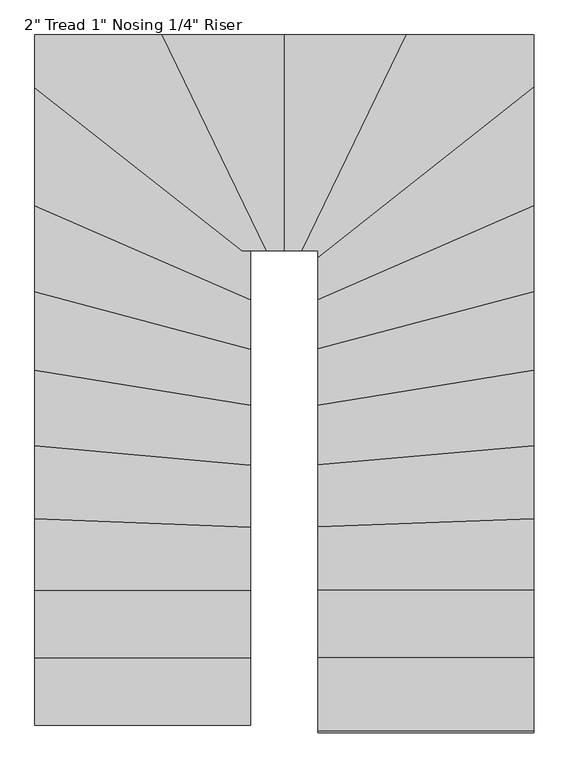
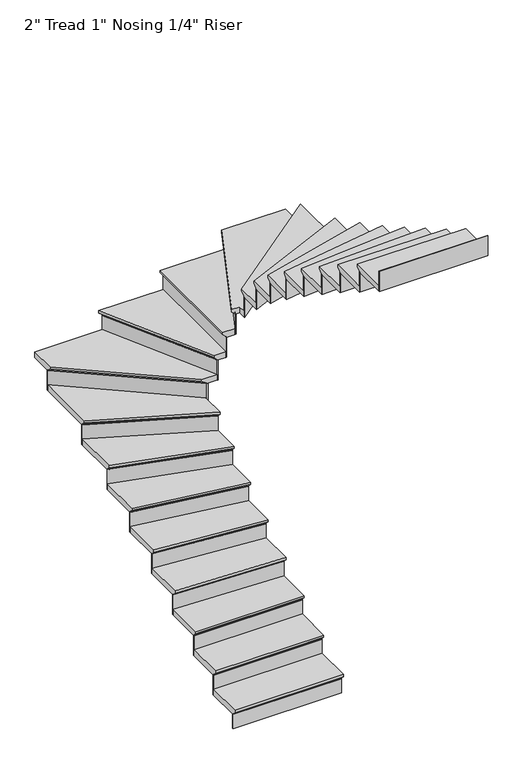
"""IFC4 building model written with IfcOpenShell, lengths in millimetres: stair flight geometry."""

from ifc_helpers import new_model, si_unit, origin, place, context, project, spatial, faceted_brep, source, transform, mapped, element, save


def stair_flight_11ab74ad(model_context):
    return source(origin(), model_context, "Body", "Brep", [
        faceted_brep([(-5047.1987704, -4554.2130548, 51361.5214286), (-5047.1987704, -4554.2130548, 51380.5714286), (-5940.8822214, -4554.2130548, 51380.5714286), (-5940.8822214, -4554.2130548, 51361.5214286), (-5047.1987704, -4528.8130548, 51336.1214286), (-5940.8822214, -4528.8130548, 51336.1214286), (-5047.1987704, -4249.4130548, 51380.5714286), (-5940.8822214, -4249.4130548, 51380.5714286), (-5940.8822214, -4528.8130548, 51329.7714286), (-5940.8822214, -4249.4130548, 51329.7714286), (-5047.1987704, -4249.4130548, 51329.7714286), (-5047.1987704, -4528.8130548, 51329.7714286)], [[[0, 1, 2, 3]], [[4, 0, 3, 5]], [[2, 1, 6, 7]], [[8, 9, 10, 11]], [[2, 7, 9, 8, 5, 3]], [[8, 11, 4, 5]], [[6, 1, 0, 4, 11, 10]], [[7, 6, 10, 9]]]),
        faceted_brep([(-5047.1987704, -4528.8130548, 51329.7714286), (-5047.1987704, -4528.8130548, 51206.4), (-5047.1987704, -4522.4630548, 51206.4), (-5047.1987704, -4522.4630548, 51329.7714286), (-5940.8822214, -4528.8130548, 51329.7714286), (-5940.8822214, -4522.4630548, 51329.7714286), (-5940.8822214, -4522.4630548, 51206.4), (-5940.8822214, -4528.8130548, 51206.4)], [[[0, 1, 2, 3]], [[4, 5, 6, 7]], [[1, 0, 4, 7]], [[2, 1, 7, 6]], [[3, 2, 6, 5]], [[0, 3, 5, 4]]]),
        faceted_brep([(-5047.1987704, -4249.4130548, 51503.9428571), (-5047.1987704, -4249.4130548, 51329.7714286), (-5047.1987704, -4243.0630548, 51329.7714286), (-5047.1987704, -4243.0630548, 51503.9428571), (-5940.8822214, -4249.4130548, 51503.9428571), (-5940.8822214, -4243.0630548, 51503.9428571), (-5940.8822214, -4243.0630548, 51329.7714286), (-5940.8822214, -4249.4130548, 51329.7714286)], [[[0, 1, 2, 3]], [[4, 5, 6, 7]], [[1, 0, 4, 7]], [[2, 1, 7, 6]], [[3, 2, 6, 5]], [[0, 3, 5, 4]]]),
        faceted_brep([(-5940.8822214, -4274.8130548, 51554.7428571), (-5047.1987704, -4274.8130548, 51554.7428571), (-5047.1987704, -3970.0130548, 51554.7428571), (-5940.8822214, -3970.0130548, 51554.7428571), (-5940.8822214, -4249.4130548, 51503.9428571), (-5940.8822214, -3970.0130548, 51503.9428571), (-5047.1987704, -3970.0130548, 51503.9428571), (-5047.1987704, -4249.4130548, 51503.9428571), (-5940.8822214, -4249.4130548, 51510.2928571), (-5940.8822214, -4274.8130548, 51535.6928571), (-5047.1987704, -4249.4130548, 51510.2928571), (-5047.1987704, -4274.8130548, 51535.6928571)], [[[0, 1, 2, 3]], [[4, 5, 6, 7]], [[0, 3, 5, 4, 8, 9]], [[4, 7, 10, 8]], [[2, 1, 11, 10, 7, 6]], [[3, 2, 6, 5]], [[11, 1, 0, 9]], [[10, 11, 9, 8]]]),
        faceted_brep([(-5047.1987704, -3970.0130548, 51678.1142857), (-5047.1987704, -3970.0130548, 51503.9428571), (-5047.1987704, -3963.6630548, 51503.9428571), (-5047.1987704, -3963.6630548, 51678.1142857), (-5940.8822214, -3970.0130548, 51678.1142857), (-5940.8822214, -3963.6630548, 51678.1142857), (-5940.8822214, -3963.6630548, 51503.9428571), (-5940.8822214, -3970.0130548, 51503.9428571)], [[[0, 1, 2, 3]], [[4, 5, 6, 7]], [[1, 0, 4, 7]], [[2, 1, 7, 6]], [[3, 2, 6, 5]], [[0, 3, 5, 4]]]),
        faceted_brep([(-5940.8822214, -3995.4130548, 51728.9142857), (-5047.1987704, -3995.4130548, 51728.9142857), (-5047.1987704, -3707.9036879, 51728.9142857), (-5940.8822214, -3673.2843203, 51728.9142857), (-5940.8822214, -3970.0130548, 51678.1142857), (-5940.8822214, -3673.2843203, 51678.1142857), (-5047.1987704, -3707.9036879, 51678.1142857), (-5047.1987704, -3970.0130548, 51678.1142857), (-5940.8822214, -3970.0130548, 51684.4642857), (-5940.8822214, -3995.4130548, 51709.8642857), (-5047.1987704, -3970.0130548, 51684.4642857), (-5047.1987704, -3995.4130548, 51709.8642857)], [[[0, 1, 2, 3]], [[4, 5, 6, 7]], [[0, 3, 5, 4, 8, 9]], [[4, 7, 10, 8]], [[2, 1, 11, 10, 7, 6]], [[3, 2, 6, 5]], [[11, 1, 0, 9]], [[10, 11, 9, 8]]]),
        faceted_brep([(-5047.1987704, -3707.9036879, 51852.2857143), (-5047.1987704, -3707.9036879, 51678.1142857), (-5047.1987704, -3701.5489252, 51678.1142857), (-5047.1987704, -3701.5489252, 51852.2857143), (-5940.8822214, -3673.2843203, 51852.2857143), (-5940.8822214, -3666.9295576, 51852.2857143), (-5940.8822214, -3666.9295576, 51678.1142857), (-5940.8822214, -3673.2843203, 51678.1142857)], [[[0, 1, 2, 3]], [[4, 5, 6, 7]], [[1, 0, 4, 7]], [[2, 1, 7, 6]], [[3, 2, 6, 5]], [[0, 3, 5, 4]]]),
        faceted_brep([(-5940.8822214, -3698.703371, 51903.0857143), (-5047.1987704, -3733.3227386, 51903.0857143), (-5047.1987704, -3451.3234819, 51903.0857143), (-5940.8822214, -3370.89733, 51903.0857143), (-5940.8822214, -3673.2843203, 51852.2857143), (-5940.8822214, -3370.89733, 51852.2857143), (-5047.1987704, -3451.3234819, 51852.2857143), (-5047.1987704, -3707.9036879, 51852.2857143), (-5940.8822214, -3673.2843203, 51858.6357143), (-5940.8822214, -3698.703371, 51884.0357143), (-5047.1987704, -3707.9036879, 51858.6357143), (-5047.1987704, -3733.3227386, 51884.0357143)], [[[0, 1, 2, 3]], [[4, 5, 6, 7]], [[0, 3, 5, 4, 8, 9]], [[4, 7, 10, 8]], [[2, 1, 11, 10, 7, 6]], [[3, 2, 6, 5]], [[11, 1, 0, 9]], [[10, 11, 9, 8]]]),
        faceted_brep([(-5047.1987704, -3451.3234819, 52026.4571429), (-5047.1987704, -3451.3234819, 51852.2857143), (-5047.1987704, -3444.9478197, 51852.2857143), (-5047.1987704, -3444.9478197, 52026.4571429), (-5940.8822214, -3370.89733, 52026.4571429), (-5940.8822214, -3364.5216678, 52026.4571429), (-5940.8822214, -3364.5216678, 51852.2857143), (-5940.8822214, -3370.89733, 51852.2857143)], [[[0, 1, 2, 3]], [[4, 5, 6, 7]], [[1, 0, 4, 7]], [[2, 1, 7, 6]], [[3, 2, 6, 5]], [[0, 3, 5, 4]]]),
        faceted_brep([(-5940.8822214, -3396.3999789, 52077.2571429), (-5047.1987704, -3476.8261308, 52077.2571429), (-5047.1987704, -3203.4301079, 52077.2571429), (-5940.8822214, -3059.5417727, 52077.2571429), (-5940.8822214, -3370.89733, 52026.4571429), (-5940.8822214, -3059.5417727, 52026.4571429), (-5047.1987704, -3203.4301079, 52026.4571429), (-5047.1987704, -3451.3234819, 52026.4571429), (-5940.8822214, -3370.89733, 52032.8071429), (-5940.8822214, -3396.3999789, 52058.2071429), (-5047.1987704, -3451.3234819, 52032.8071429), (-5047.1987704, -3476.8261308, 52058.2071429)], [[[0, 1, 2, 3]], [[4, 5, 6, 7]], [[0, 3, 5, 4, 8, 9]], [[4, 7, 10, 8]], [[2, 1, 11, 10, 7, 6]], [[3, 2, 6, 5]], [[11, 1, 0, 9]], [[10, 11, 9, 8]]]),
        faceted_brep([(-5047.1987704, -3203.4301079, 52200.6285714), (-5047.1987704, -3203.4301079, 52026.4571429), (-5047.1987704, -3196.9983292, 52026.4571429), (-5047.1987704, -3196.9983292, 52200.6285714), (-5940.8822214, -3059.5417727, 52200.6285714), (-5940.8822214, -3053.109994, 52200.6285714), (-5940.8822214, -3053.109994, 52026.4571429), (-5940.8822214, -3059.5417727, 52026.4571429)], [[[0, 1, 2, 3]], [[4, 5, 6, 7]], [[1, 0, 4, 7]], [[2, 1, 7, 6]], [[3, 2, 6, 5]], [[0, 3, 5, 4]]]),
        faceted_brep([(-5940.8822214, -3085.2688872, 52251.4285714), (-5047.1987704, -3229.1572224, 52251.4285714), (-5047.1987704, -2970.3553609, 52251.4285714), (-5940.8822214, -2732.7052783, 52251.4285714), (-5940.8822214, -3059.5417727, 52200.6285714), (-5940.8822214, -2732.7052783, 52200.6285714), (-5047.1987704, -2970.3553609, 52200.6285714), (-5047.1987704, -3203.4301079, 52200.6285714), (-5940.8822214, -3059.5417727, 52206.9785714), (-5940.8822214, -3085.2688872, 52232.3785714), (-5047.1987704, -3203.4301079, 52206.9785714), (-5047.1987704, -3229.1572224, 52232.3785714)], [[[0, 1, 2, 3]], [[4, 5, 6, 7]], [[0, 3, 5, 4, 8, 9]], [[4, 7, 10, 8]], [[2, 1, 11, 10, 7, 6]], [[3, 2, 6, 5]], [[11, 1, 0, 9]], [[10, 11, 9, 8]]]),
        faceted_brep([(-5047.1987704, -2970.3553609, 52374.8), (-5047.1987704, -2970.3553609, 52200.6285714), (-5047.1987704, -2963.7846771, 52200.6285714), (-5047.1987704, -2963.7846771, 52374.8), (-5940.8822214, -2732.7052783, 52374.8), (-5940.8822214, -2726.1345945, 52374.8), (-5940.8822214, -2726.1345945, 52200.6285714), (-5940.8822214, -2732.7052783, 52200.6285714)], [[[0, 1, 2, 3]], [[4, 5, 6, 7]], [[1, 0, 4, 7]], [[2, 1, 7, 6]], [[3, 2, 6, 5]], [[0, 3, 5, 4]]]),
        faceted_brep([(-5940.8822214, -2758.9880136, 52425.6), (-5047.1987704, -2996.6380961, 52425.6), (-5047.1987704, -2765.8050203, 52425.6), (-5940.8822214, -2375.5896532, 52425.6), (-5940.8822214, -2732.7052783, 52374.8), (-5940.8822214, -2375.5896532, 52374.8), (-5047.1987704, -2765.8050203, 52374.8), (-5047.1987704, -2970.3553609, 52374.8), (-5940.8822214, -2732.7052783, 52381.15), (-5940.8822214, -2758.9880136, 52406.55), (-5047.1987704, -2970.3553609, 52381.15), (-5047.1987704, -2996.6380961, 52406.55)], [[[0, 1, 2, 3]], [[4, 5, 6, 7]], [[0, 3, 5, 4, 8, 9]], [[4, 7, 10, 8]], [[2, 1, 11, 10, 7, 6]], [[3, 2, 6, 5]], [[11, 1, 0, 9]], [[10, 11, 9, 8]]]),
        faceted_brep([(-5047.1987704, -2765.8050203, 52548.9714286), (-5047.1987704, -2765.8050203, 52374.8), (-5047.1987704, -2758.8760908, 52374.8), (-5047.1987704, -2758.8760908, 52548.9714286), (-5940.8822214, -2375.5896532, 52548.9714286), (-5940.8822214, -2368.6607237, 52548.9714286), (-5940.8822214, -2368.6607237, 52374.8), (-5940.8822214, -2375.5896532, 52374.8)], [[[0, 1, 2, 3]], [[4, 5, 6, 7]], [[1, 0, 4, 7]], [[2, 1, 7, 6]], [[3, 2, 6, 5]], [[0, 3, 5, 4]]]),
        faceted_brep([(-5940.8822214, -2403.3053713, 52599.7714286), (-5047.1987704, -2793.5207384, 52599.7714286), (-5047.1987704, -2590.8424524, 52599.7714286), (-5040.8038639, -2590.8424524, 52599.7714286), (-5940.8822214, -1882.1944717, 52599.7714286), (-5940.8822214, -2375.5896532, 52548.9714286), (-5940.8822214, -1882.1944717, 52548.9714286), (-5040.8038639, -2590.8424524, 52548.9714286), (-5047.1987704, -2590.8424524, 52548.9714286), (-5047.1987704, -2765.8050203, 52548.9714286), (-5940.8822214, -2375.5896532, 52555.3214286), (-5940.8822214, -2403.3053713, 52580.7214286), (-5047.1987704, -2765.8050203, 52555.3214286), (-5047.1987704, -2793.5207384, 52580.7214286)], [[[0, 1, 2, 3, 4]], [[5, 6, 7, 8, 9]], [[0, 4, 6, 5, 10, 11]], [[5, 9, 12, 10]], [[2, 1, 13, 12, 9, 8]], [[4, 3, 7, 6]], [[13, 1, 0, 11]], [[12, 13, 11, 10]], [[3, 2, 8, 7]]]),
        faceted_brep([(-5040.8038639, -2590.8424524, 52723.1428571), (-5040.8038639, -2590.8424524, 52548.9714286), (-5030.5387554, -2590.8424524, 52548.9714286), (-5030.5387554, -2590.8424524, 52723.1428571), (-5940.8822214, -1882.1944717, 52723.1428571), (-5940.8822214, -1874.1125661, 52723.1428571), (-5940.8822214, -1874.1125661, 52548.9714286), (-5940.8822214, -1882.1944717, 52548.9714286)], [[[0, 1, 2, 3]], [[4, 5, 6, 7]], [[1, 0, 4, 7]], [[2, 1, 7, 6]], [[3, 2, 6, 5]], [[0, 3, 5, 4]]]),
        faceted_brep([(-5384.6489457, -1697.1590014, 52773.9428571), (-5940.8822214, -1697.1590014, 52773.9428571), (-5940.8822214, -1914.5220945, 52773.9428571), (-5081.8642978, -2590.8424524, 52773.9428571), (-4952.3566185, -2590.8424524, 52773.9428571), (-5940.8822214, -1697.1590014, 52723.1428571), (-5384.6489457, -1697.1590014, 52723.1428571), (-4952.3566185, -2590.8424524, 52723.1428571), (-5040.8038639, -2590.8424524, 52723.1428571), (-5940.8822214, -1882.1944717, 52723.1428571), (-5940.8822214, -1882.1944717, 52729.4928571), (-5940.8822214, -1914.5220945, 52754.8928571), (-5040.8038639, -2590.8424524, 52729.4928571), (-5081.8642978, -2590.8424524, 52754.8928571)], [[[0, 1, 2, 3, 4]], [[5, 6, 7, 8, 9]], [[1, 0, 6, 5]], [[2, 1, 5, 9, 10, 11]], [[9, 8, 12, 10]], [[4, 3, 13, 12, 8, 7]], [[0, 4, 7, 6]], [[13, 3, 2, 11]], [[12, 13, 11, 10]]]),
        faceted_brep([(-4952.3566185, -2590.8424524, 52897.3142857), (-4952.3566185, -2590.8424524, 52723.1428571), (-4945.3027294, -2590.8424524, 52723.1428571), (-4945.3027294, -2590.8424524, 52897.3142857), (-5384.6489457, -1697.1590014, 52897.3142857), (-5377.5950566, -1697.1590014, 52897.3142857), (-5377.5950566, -1697.1590014, 52723.1428571), (-5384.6489457, -1697.1590014, 52723.1428571)], [[[0, 1, 2, 3]], [[4, 5, 6, 7]], [[1, 0, 4, 7]], [[2, 1, 7, 6]], [[3, 2, 6, 5]], [[0, 3, 5, 4]]]),
        faceted_brep([(-5412.8645022, -1697.1590014, 52948.1142857), (-4980.5721749, -2590.8424524, 52948.1142857), (-4882.0987704, -2590.8424524, 52948.1142857), (-4882.0987706, -1697.1590014, 52948.1142857), (-5384.6489457, -1697.1590014, 52897.3142857), (-4882.0987706, -1697.1590014, 52897.3142857), (-4882.0987704, -2590.8424524, 52897.3142857), (-4952.3566185, -2590.8424524, 52897.3142857), (-5384.6489457, -1697.1590014, 52903.6642857), (-5412.8645022, -1697.1590014, 52929.0642857), (-4952.3566185, -2590.8424524, 52903.6642857), (-4980.5721749, -2590.8424524, 52929.0642857)], [[[0, 1, 2, 3]], [[4, 5, 6, 7]], [[0, 3, 5, 4, 8, 9]], [[4, 7, 10, 8]], [[3, 2, 6, 5]], [[11, 1, 0, 9]], [[10, 11, 9, 8]], [[2, 1, 11, 10, 7, 6]]]),
        faceted_brep([(-4882.0987704, -2590.8424524, 53071.4857143), (-4882.0987704, -2590.8424524, 52897.3142857), (-4875.7487704, -2590.8424524, 52897.3142857), (-4875.7487704, -2590.8424524, 53071.4857143), (-4882.0987706, -1697.1590014, 53071.4857143), (-4875.7487706, -1697.1590014, 53071.4857143), (-4875.7487706, -1697.1590014, 52897.3142857), (-4882.0987706, -1697.1590014, 52897.3142857)], [[[0, 1, 2, 3]], [[4, 5, 6, 7]], [[1, 0, 4, 7]], [[2, 1, 7, 6]], [[3, 2, 6, 5]], [[0, 3, 5, 4]]]),
        faceted_brep([(-4907.4987706, -1697.1590014, 53122.2857143), (-4907.4987704, -2590.8424524, 53122.2857143), (-4806.2098095, -2590.8424524, 53122.2857143), (-4373.9174828, -1697.1590014, 53122.2857143), (-4882.0987706, -1697.1590014, 53071.4857143), (-4373.9174828, -1697.1590014, 53071.4857143), (-4806.2098095, -2590.8424524, 53071.4857143), (-4882.0987704, -2590.8424524, 53071.4857143), (-4882.0987706, -1697.1590014, 53077.8357143), (-4907.4987706, -1697.1590014, 53103.2357143), (-4882.0987704, -2590.8424524, 53077.8357143), (-4907.4987704, -2590.8424524, 53103.2357143)], [[[0, 1, 2, 3]], [[4, 5, 6, 7]], [[0, 3, 5, 4, 8, 9]], [[4, 7, 10, 8]], [[2, 1, 11, 10, 7, 6]], [[3, 2, 6, 5]], [[11, 1, 0, 9]], [[10, 11, 9, 8]]]),
        faceted_brep([(-4806.2098095, -2590.8424524, 53245.6571429), (-4806.2098095, -2590.8424524, 53071.4857143), (-4799.1559204, -2590.8424524, 53071.4857143), (-4799.1559204, -2590.8424524, 53245.6571429), (-4373.9174828, -1697.1590014, 53245.6571429), (-4366.8635937, -1697.1590014, 53245.6571429), (-4366.8635937, -1697.1590014, 53071.4857143), (-4373.9174828, -1697.1590014, 53071.4857143)], [[[0, 1, 2, 3]], [[4, 5, 6, 7]], [[1, 0, 4, 7]], [[2, 1, 7, 6]], [[3, 2, 6, 5]], [[0, 3, 5, 4]]]),
        faceted_brep([(-3874.1153195, -1946.8497166, 53296.4571429), (-3874.1153195, -1697.1590014, 53296.4571429), (-4402.1330392, -1697.1590014, 53296.4571429), (-4834.4253659, -2590.8424524, 53296.4571429), (-4767.7987704, -2590.8424524, 53296.4571429), (-4767.7987704, -2650.4628721, 53296.4571429), (-3874.1153195, -1697.1590014, 53245.6571429), (-3874.1153195, -1946.8497166, 53245.6571429), (-4767.7987704, -2650.4628721, 53245.6571429), (-4767.7987704, -2590.8424524, 53245.6571429), (-4806.2098095, -2590.8424524, 53245.6571429), (-4373.9174828, -1697.1590014, 53245.6571429), (-4806.2098095, -2590.8424524, 53252.0071429), (-4373.9174828, -1697.1590014, 53252.0071429), (-4834.4253659, -2590.8424524, 53277.4071429), (-4402.1330392, -1697.1590014, 53277.4071429)], [[[0, 1, 2, 3, 4, 5]], [[6, 7, 8, 9, 10, 11]], [[1, 0, 7, 6]], [[11, 10, 12, 13]], [[4, 3, 14, 12, 10, 9]], [[5, 4, 9, 8]], [[0, 5, 8, 7]], [[14, 3, 2, 15]], [[12, 14, 15, 13]], [[2, 1, 6, 11, 13, 15]]]),
        faceted_brep([(-4767.7987704, -2650.4628721, 53419.8285714), (-4767.7987704, -2650.4628721, 53245.6571429), (-4767.7987704, -2658.5447778, 53245.6571429), (-4767.7987704, -2658.5447778, 53419.8285714), (-3874.1153195, -1946.8497166, 53419.8285714), (-3874.1153195, -1954.9316222, 53419.8285714), (-3874.1153195, -1954.9316222, 53245.6571429), (-3874.1153195, -1946.8497166, 53245.6571429)], [[[0, 1, 2, 3]], [[4, 5, 6, 7]], [[1, 0, 4, 7]], [[2, 1, 7, 6]], [[3, 2, 6, 5]], [[0, 3, 5, 4]]]),
        faceted_brep([(-3874.1153195, -1914.5220938, 53470.6285714), (-4767.7987704, -2618.1352494, 53470.6285714), (-4767.7987704, -2821.2364563, 53470.6285714), (-3874.1153195, -2431.0210889, 53470.6285714), (-3874.1153195, -1946.8497166, 53419.8285714), (-3874.1153195, -2431.0210889, 53419.8285714), (-4767.7987704, -2821.2364563, 53419.8285714), (-4767.7987704, -2650.4628721, 53419.8285714), (-3874.1153195, -1946.8497166, 53426.1785714), (-3874.1153195, -1914.5220938, 53451.5785714), (-4767.7987704, -2650.4628721, 53426.1785714), (-4767.7987704, -2618.1352494, 53451.5785714)], [[[0, 1, 2, 3]], [[4, 5, 6, 7]], [[0, 3, 5, 4, 8, 9]], [[4, 7, 10, 8]], [[2, 1, 11, 10, 7, 6]], [[3, 2, 6, 5]], [[11, 1, 0, 9]], [[10, 11, 9, 8]]]),
        faceted_brep([(-4767.7987704, -2821.2364563, 53594.0), (-4767.7987704, -2821.2364563, 53419.8285714), (-4767.7987704, -2828.1653858, 53419.8285714), (-4767.7987704, -2828.1653858, 53594.0), (-3874.1153195, -2431.0210889, 53594.0), (-3874.1153195, -2437.9500185, 53594.0), (-3874.1153195, -2437.9500185, 53419.8285714), (-3874.1153195, -2431.0210889, 53419.8285714)], [[[0, 1, 2, 3]], [[4, 5, 6, 7]], [[1, 0, 4, 7]], [[2, 1, 7, 6]], [[3, 2, 6, 5]], [[0, 3, 5, 4]]]),
        faceted_brep([(-3874.1153195, -2403.3053709, 53644.8), (-4767.7987704, -2793.5207382, 53644.8), (-4767.7987704, -3022.9208311, 53644.8), (-3874.1153195, -2785.2707484, 53644.8), (-3874.1153195, -2431.0210889, 53594.0), (-3874.1153195, -2785.2707484, 53594.0), (-4767.7987704, -3022.9208311, 53594.0), (-4767.7987704, -2821.2364563, 53594.0), (-3874.1153195, -2431.0210889, 53600.35), (-3874.1153195, -2403.3053709, 53625.75), (-4767.7987704, -2821.2364563, 53600.35), (-4767.7987704, -2793.5207382, 53625.75)], [[[0, 1, 2, 3]], [[4, 5, 6, 7]], [[0, 3, 5, 4, 8, 9]], [[4, 7, 10, 8]], [[2, 1, 11, 10, 7, 6]], [[3, 2, 6, 5]], [[11, 1, 0, 9]], [[10, 11, 9, 8]]]),
        faceted_brep([(-4767.7987704, -3022.9208311, 53768.1714286), (-4767.7987704, -3022.9208311, 53594.0), (-4767.7987704, -3029.4915149, 53594.0), (-4767.7987704, -3029.4915149, 53768.1714286), (-3874.1153195, -2785.2707484, 53768.1714286), (-3874.1153195, -2791.8414322, 53768.1714286), (-3874.1153195, -2791.8414322, 53594.0), (-3874.1153195, -2785.2707484, 53594.0)], [[[0, 1, 2, 3]], [[4, 5, 6, 7]], [[1, 0, 4, 7]], [[2, 1, 7, 6]], [[3, 2, 6, 5]], [[0, 3, 5, 4]]]),
        faceted_brep([(-3874.1153195, -2758.9880132, 53818.9714286), (-4767.7987704, -2996.6380959, 53818.9714286), (-4767.7987704, -3254.8843368, 53818.9714286), (-3874.1153195, -3110.9960015, 53818.9714286), (-3874.1153195, -2785.2707484, 53768.1714286), (-3874.1153195, -3110.9960015, 53768.1714286), (-4767.7987704, -3254.8843368, 53768.1714286), (-4767.7987704, -3022.9208311, 53768.1714286), (-3874.1153195, -2785.2707484, 53774.5214286), (-3874.1153195, -2758.9880132, 53799.9214286), (-4767.7987704, -3022.9208311, 53774.5214286), (-4767.7987704, -2996.6380959, 53799.9214286)], [[[0, 1, 2, 3]], [[4, 5, 6, 7]], [[0, 3, 5, 4, 8, 9]], [[4, 7, 10, 8]], [[2, 1, 11, 10, 7, 6]], [[3, 2, 6, 5]], [[11, 1, 0, 9]], [[10, 11, 9, 8]]]),
        faceted_brep([(-4767.7987704, -3254.8843368, 53942.3428571), (-4767.7987704, -3254.8843368, 53768.1714286), (-4767.7987704, -3261.3161154, 53768.1714286), (-4767.7987704, -3261.3161154, 53942.3428571), (-3874.1153195, -3110.9960015, 53942.3428571), (-3874.1153195, -3117.4277801, 53942.3428571), (-3874.1153195, -3117.4277801, 53768.1714286), (-3874.1153195, -3110.9960015, 53768.1714286)], [[[0, 1, 2, 3]], [[4, 5, 6, 7]], [[1, 0, 4, 7]], [[2, 1, 7, 6]], [[3, 2, 6, 5]], [[0, 3, 5, 4]]]),
        faceted_brep([(-3874.1153195, -3085.2688869, 53993.1428571), (-4767.7987704, -3229.1572222, 53993.1428571), (-4767.7987704, -3502.3287795, 53993.1428571), (-3874.1153195, -3421.9026274, 53993.1428571), (-3874.1153195, -3110.9960015, 53942.3428571), (-3874.1153195, -3421.9026274, 53942.3428571), (-4767.7987704, -3502.3287795, 53942.3428571), (-4767.7987704, -3254.8843368, 53942.3428571), (-3874.1153195, -3110.9960015, 53948.6928571), (-3874.1153195, -3085.2688869, 53974.0928571), (-4767.7987704, -3254.8843368, 53948.6928571), (-4767.7987704, -3229.1572222, 53974.0928571)], [[[0, 1, 2, 3]], [[4, 5, 6, 7]], [[0, 3, 5, 4, 8, 9]], [[4, 7, 10, 8]], [[2, 1, 11, 10, 7, 6]], [[3, 2, 6, 5]], [[11, 1, 0, 9]], [[10, 11, 9, 8]]]),
        faceted_brep([(-4767.7987704, -3502.3287795, 54116.5142857), (-4767.7987704, -3502.3287795, 53942.3428571), (-4767.7987704, -3508.7044417, 53942.3428571), (-4767.7987704, -3508.7044417, 54116.5142857), (-3874.1153195, -3421.9026274, 54116.5142857), (-3874.1153195, -3428.2782897, 54116.5142857), (-3874.1153195, -3428.2782897, 53942.3428571), (-3874.1153195, -3421.9026274, 53942.3428571)], [[[0, 1, 2, 3]], [[4, 5, 6, 7]], [[1, 0, 4, 7]], [[2, 1, 7, 6]], [[3, 2, 6, 5]], [[0, 3, 5, 4]]]),
        faceted_brep([(-3874.1153195, -3396.3999786, 54167.3142857), (-4767.7987704, -3476.8261306, 54167.3142857), (-4767.7987704, -3758.7417891, 54167.3142857), (-3874.1153195, -3724.1224215, 54167.3142857), (-3874.1153195, -3421.9026274, 54116.5142857), (-3874.1153195, -3724.1224215, 54116.5142857), (-4767.7987704, -3758.7417891, 54116.5142857), (-4767.7987704, -3502.3287795, 54116.5142857), (-3874.1153195, -3421.9026274, 54122.8642857), (-3874.1153195, -3396.3999786, 54148.2642857), (-4767.7987704, -3502.3287795, 54122.8642857), (-4767.7987704, -3476.8261306, 54148.2642857)], [[[0, 1, 2, 3]], [[4, 5, 6, 7]], [[0, 3, 5, 4, 8, 9]], [[4, 7, 10, 8]], [[2, 1, 11, 10, 7, 6]], [[3, 2, 6, 5]], [[11, 1, 0, 9]], [[10, 11, 9, 8]]]),
        faceted_brep([(-4767.7987704, -3758.7417891, 54290.6857143), (-4767.7987704, -3758.7417891, 54116.5142857), (-4767.7987704, -3765.0965518, 54116.5142857), (-4767.7987704, -3765.0965518, 54290.6857143), (-3874.1153195, -3724.1224215, 54290.6857143), (-3874.1153195, -3730.4771842, 54290.6857143), (-3874.1153195, -3730.4771842, 54116.5142857), (-3874.1153195, -3724.1224215, 54116.5142857)], [[[0, 1, 2, 3]], [[4, 5, 6, 7]], [[1, 0, 4, 7]], [[2, 1, 7, 6]], [[3, 2, 6, 5]], [[0, 3, 5, 4]]]),
        faceted_brep([(-3874.1153195, -3698.7033708, 54341.4857143), (-4767.7987704, -3733.3227384, 54341.4857143), (-4767.7987704, -4020.8130546, 54341.4857143), (-3874.1153195, -4020.8130546, 54341.4857143), (-3874.1153195, -3724.1224215, 54290.6857143), (-3874.1153195, -4020.8130546, 54290.6857143), (-4767.7987704, -4020.8130546, 54290.6857143), (-4767.7987704, -3758.7417891, 54290.6857143), (-3874.1153195, -3724.1224215, 54297.0357143), (-3874.1153195, -3698.7033708, 54322.4357143), (-4767.7987704, -3758.7417891, 54297.0357143), (-4767.7987704, -3733.3227384, 54322.4357143)], [[[0, 1, 2, 3]], [[4, 5, 6, 7]], [[0, 3, 5, 4, 8, 9]], [[4, 7, 10, 8]], [[2, 1, 11, 10, 7, 6]], [[3, 2, 6, 5]], [[11, 1, 0, 9]], [[10, 11, 9, 8]]]),
        faceted_brep([(-4767.7987704, -4020.8130546, 54464.8571429), (-4767.7987704, -4020.8130546, 54290.6857143), (-4767.7987704, -4027.1630546, 54290.6857143), (-4767.7987704, -4027.1630546, 54464.8571429), (-3874.1153195, -4020.8130546, 54464.8571429), (-3874.1153195, -4027.1630546, 54464.8571429), (-3874.1153195, -4027.1630546, 54290.6857143), (-3874.1153195, -4020.8130546, 54290.6857143)], [[[0, 1, 2, 3]], [[4, 5, 6, 7]], [[1, 0, 4, 7]], [[2, 1, 7, 6]], [[3, 2, 6, 5]], [[0, 3, 5, 4]]]),
        faceted_brep([(-3874.1153195, -3995.4130546, 54515.6571429), (-4767.7987704, -3995.4130546, 54515.6571429), (-4767.7987704, -4300.2130546, 54515.6571429), (-3874.1153195, -4300.2130546, 54515.6571429), (-3874.1153195, -4020.8130546, 54464.8571429), (-3874.1153195, -4300.2130546, 54464.8571429), (-4767.7987704, -4300.2130546, 54464.8571429), (-4767.7987704, -4020.8130546, 54464.8571429), (-3874.1153195, -4020.8130546, 54471.2071429), (-3874.1153195, -3995.4130546, 54496.6071429), (-4767.7987704, -4020.8130546, 54471.2071429), (-4767.7987704, -3995.4130546, 54496.6071429)], [[[0, 1, 2, 3]], [[4, 5, 6, 7]], [[0, 3, 5, 4, 8, 9]], [[4, 7, 10, 8]], [[2, 1, 11, 10, 7, 6]], [[3, 2, 6, 5]], [[11, 1, 0, 9]], [[10, 11, 9, 8]]]),
        faceted_brep([(-4767.7987704, -4300.2130546, 54639.0285714), (-4767.7987704, -4300.2130546, 54464.8571429), (-4767.7987704, -4306.5630546, 54464.8571429), (-4767.7987704, -4306.5630546, 54639.0285714), (-3874.1153195, -4300.2130546, 54639.0285714), (-3874.1153195, -4306.5630546, 54639.0285714), (-3874.1153195, -4306.5630546, 54464.8571429), (-3874.1153195, -4300.2130546, 54464.8571429)], [[[0, 1, 2, 3]], [[4, 5, 6, 7]], [[1, 0, 4, 7]], [[2, 1, 7, 6]], [[3, 2, 6, 5]], [[0, 3, 5, 4]]]),
        faceted_brep([(-4767.7987704, -4579.6130546, 54813.2), (-4767.7987704, -4579.6130546, 54639.0285714), (-4767.7987704, -4585.9630546, 54639.0285714), (-4767.7987704, -4585.9630546, 54813.2), (-3874.1153195, -4579.6130546, 54813.2), (-3874.1153195, -4585.9630546, 54813.2), (-3874.1153195, -4585.9630546, 54639.0285714), (-3874.1153195, -4579.6130546, 54639.0285714)], [[[0, 1, 2, 3]], [[4, 5, 6, 7]], [[1, 0, 4, 7]], [[2, 1, 7, 6]], [[3, 2, 6, 5]], [[0, 3, 5, 4]]]),
        faceted_brep([(-3874.1153195, -4274.8130546, 54689.8285714), (-4767.7987704, -4274.8130546, 54689.8285714), (-4767.7987704, -4579.6130546, 54689.8285714), (-3874.1153195, -4579.6130546, 54689.8285714), (-3874.1153195, -4300.2130546, 54639.0285714), (-3874.1153195, -4579.6130546, 54639.0285714), (-4767.7987704, -4579.6130546, 54639.0285714), (-4767.7987704, -4300.2130546, 54639.0285714), (-3874.1153195, -4300.2130546, 54645.3785714), (-3874.1153195, -4274.8130546, 54670.7785714), (-4767.7987704, -4300.2130546, 54645.3785714), (-4767.7987704, -4274.8130546, 54670.7785714)], [[[0, 1, 2, 3]], [[4, 5, 6, 7]], [[0, 3, 5, 4, 8, 9]], [[4, 7, 10, 8]], [[2, 1, 11, 10, 7, 6]], [[3, 2, 6, 5]], [[11, 1, 0, 9]], [[10, 11, 9, 8]]]),
    ])


if __name__ == "__main__":
    model = new_model("IFC4")
    model_context = context("Model", 3, world=origin())
    ifc_project = project(units=[si_unit("LENGTHUNIT", "METRE", prefix="MILLI")], contexts=[model_context])
    site = spatial("IfcSite", under=ifc_project)
    building = spatial("IfcBuilding", under=site)
    placement = place(None, origin())
    stair_flight_shape = stair_flight_11ab74ad(model_context)
    element("IfcStairFlight", 1, ObjectType="2\" Tread 1\" Nosing 1/4\" Riser", at=placement, inside=building, context=model_context, shape_type="MappedRepresentation", body=[
        mapped(stair_flight_shape, transform((0.0, 0.0, 0.0), x_axis=(1.0, 0.0, 0.0), y_axis=(0.0, 1.0, 0.0), z_axis=(0.0, 0.0, 1.0))),
    ])
    save(model, "model.ifc")

# Revit data of these elements
# Element 1 (IfcStairFlight, "2\" Tread 1\" Nosing 1/4\" Riser")
#   Materials on its faces: "Tile, Porcelain, 4in"
# Materials
#   "Tile, Porcelain, 4in": class "Generic", colour RGB 89 87 158, transparency 0, Description = "Porcelain tile, 4\", white", Cost = 0
